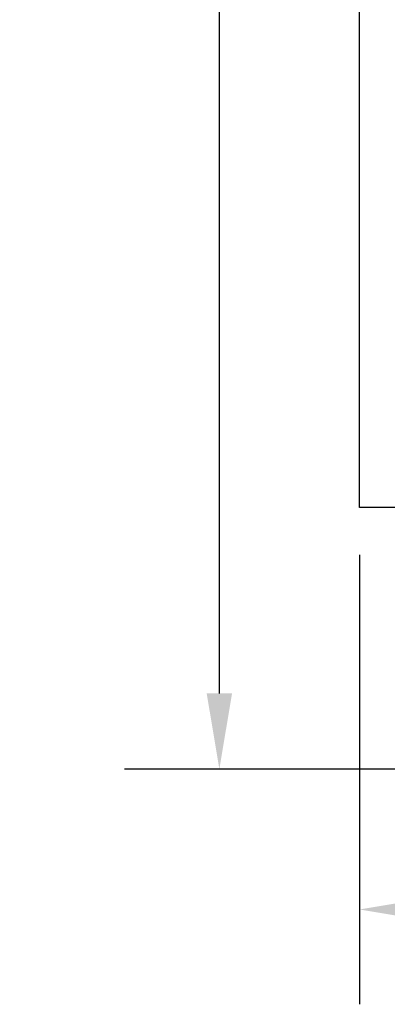
# Model space of a CAD drawing. Units: millimetres. Extents: x 7894 to 8038, y 6851 to 6951.
# Tile 1 of 49: x 7940.01 to 7944.85, y 6858.51 to 6871.49. Entities that reach past the tile are written whole.
import ezdxf

# ---------------------------------------------------------------- set-up
doc = ezdxf.new("R2010")
doc.units = ezdxf.units.MM
doc.layers.add('A-ANNO-DIMS', color=2, linetype='Continuous', lineweight=18)
doc.layers.add('A-FURN-CASE', color=7, linetype='Continuous', lineweight=30)
doc.styles.get("Standard").update_dxf_attribs({"font": 'arial.ttf'})
doc.dimstyles.new('ISO-25', dxfattribs={"dimtxt": 1, "dimasz": 1, "dimexe": 1.25, "dimexo": 0.625, "dimtad": 1, "dimdec": 0, "dimlunit": 4, "dimtxsty": 'Standard', "dimcen": 2.5, "dimclrt": 1, "dimadec": 0, "dimazin": 0, "dimtfac": 1, "dimtdec": 0, "dimtmove": 0, "dimatfit": 3, "dimfxl": 1, "dimarcsym": 0})

# ---------------------------------------------------------------- blocks, each defined once
blk = doc.blocks.new('*D36')
at = {"layer": 'A-ANNO-DIMS', "color": 0, "lineweight": -2, "transparency": 16777216}
for p, q in [((7980.836, 6877.959), (7980.836, 6858.512)), ((7944.487, 6864.436), (7944.487, 6858.512)), ((7945.487, 6859.762), (7979.836, 6859.762))]:
    blk.add_line(p, q, dxfattribs=at)
at = {"layer": 'A-ANNO-DIMS', "color": 0, "transparency": 16777216}
for points in [[(7945.487, 6859.929), (7945.487, 6859.596), (7944.487, 6859.762)], [(7979.836, 6859.929), (7979.836, 6859.596), (7980.836, 6859.762)]]:
    blk.add_solid(points, dxfattribs=at)
at = {"layer": 'Defpoints', "color": 0, "transparency": 16777216}
for p in [(7980.836, 6878.584), (7944.487, 6865.061), (7980.836, 6859.762)]:
    blk.add_point(p, dxfattribs=at)
at = {"layer": 'A-ANNO-DIMS', "color": 1, "transparency": 16777216, "insert": (7962.661, 6860.905), "char_height": 1, "attachment_point": 5}
blk.add_mtext('3\'-0 1/2"', dxfattribs=at)
blk = doc.blocks.new('*D37')
at = {"layer": 'A-ANNO-DIMS', "color": 0, "lineweight": -2, "transparency": 16777216}
for p, q in [((7954.92, 6887.903), (7941.389, 6887.903)), ((7942.639, 6862.61), (7942.639, 6886.903)), ((7953.623, 6861.61), (7941.389, 6861.61))]:
    blk.add_line(p, q, dxfattribs=at)
at = {"layer": 'A-ANNO-DIMS', "color": 0, "transparency": 16777216}
for points in [[(7942.472, 6886.903), (7942.806, 6886.903), (7942.639, 6887.903)], [(7942.472, 6862.61), (7942.806, 6862.61), (7942.639, 6861.61)]]:
    blk.add_solid(points, dxfattribs=at)
at = {"layer": 'Defpoints', "color": 0, "transparency": 16777216}
for p in [(7942.639, 6887.903), (7955.545, 6887.903), (7954.248, 6861.61)]:
    blk.add_point(p, dxfattribs=at)
at = {"layer": 'A-ANNO-DIMS', "color": 1, "transparency": 16777216, "insert": (7941.497, 6874.756), "char_height": 1, "attachment_point": 5, "rotation": 90}
blk.add_mtext('2\'-2 1/2"', dxfattribs=at)

msp = doc.modelspace()

# ---------------------------------------------------------------- linework, layer by layer
at = {"layer": 'A-FURN-CASE'}
msp.add_lwpolyline([(7944.487, 6876.461), (7955.887, 6876.461), (7955.887, 6865.061), (7944.487, 6865.061)], close=True, dxfattribs=at)

# ---------------------------------------------------------------- dimensions: what is measured, and where the dimension line sits
at = {"layer": 'A-ANNO-DIMS'}
dim = msp.add_linear_dim(base=(7942.639, 6887.903), p1=(7954.248, 6861.61), p2=(7955.545, 6887.903), angle=90, dimstyle='ISO-25', override={"dimdec": 1, "dimlfac": 1, "dimrnd": 0, "dimzin": 1, "dimdsep": 46, "dimlunit": 4, "dimfrac": 2}, dxfattribs=at)
dim.commit()
dim.dimension.update_dxf_attribs({"geometry": '*D37', "text_midpoint": (7941.497, 6874.756)})
dim = msp.add_linear_dim(base=(7980.836, 6859.762), p1=(7944.487, 6865.061), p2=(7980.836, 6878.584), dimstyle='ISO-25', override={"dimdec": 1, "dimlfac": 1, "dimrnd": 0, "dimzin": 1, "dimdsep": 46, "dimlunit": 4, "dimfrac": 2}, dxfattribs=at)
dim.commit()
dim.dimension.update_dxf_attribs({"geometry": '*D36', "text_midpoint": (7962.661, 6860.905)})

doc.saveas('drawing.dxf')
